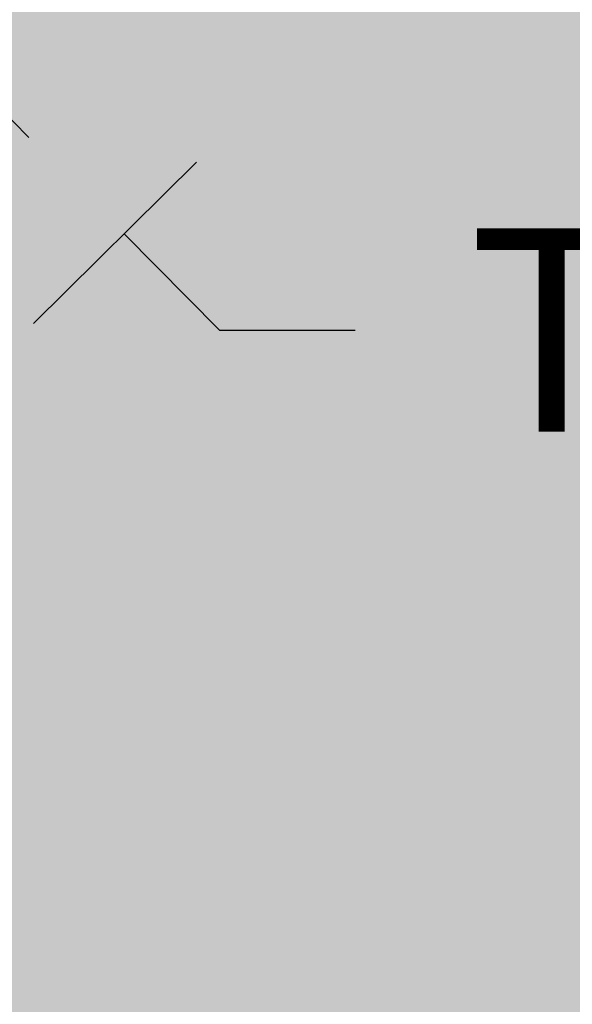
# Model space of a CAD drawing. Units: inches. Extents: x -466983 to 1020, y 324 to 318697.
# Tile 14 of 97: x 736 to 752, y 452 to 482. Entities that reach past the tile are written whole.
import ezdxf

# ---------------------------------------------------------------- set-up
doc = ezdxf.new("R2010")
doc.units = ezdxf.units.IN
doc.header["$MEASUREMENT"] = 0
doc.layers.add('A-ANNO-DIMS', color=2, linetype='Continuous', lineweight=18)
doc.layers.add('A-FLOR-PATT', color=252, linetype='Continuous', lineweight=13)
doc.styles.get("Standard").update_dxf_attribs({"font": 'arial.ttf'})
doc.dimstyles.get("Standard").update_dxf_attribs({"dimtxt": 6, "dimasz": 4, "dimexe": 3, "dimexo": 3, "dimgap": 0.09, "dimtad": 0, "dimtih": 1, "dimtoh": 1, "dimdec": 1, "dimzin": 0, "dimdsep": 46, "dimlunit": 3, "dimtxsty": 'Standard', "dimcen": 0.09, "dimadec": 0, "dimazin": 0, "dimtfac": 1, "dimtdec": 1, "dimtofl": 0, "dimtmove": 0, "dimatfit": 3, "dimfxl": 1, "dimtolj": 1, "dimtzin": 0, "dimarcsym": 0})

# ---------------------------------------------------------------- blocks, each defined once
blk = doc.blocks.new('*D113')
at = {"layer": 'A-ANNO-DIMS', "color": 0, "lineweight": -2, "transparency": 16777216}
for p, q in [((704.7099345407843, 504.6522237351473), (709.5248847709719, 509.4132675549068)), ((710.2041170385384, 504.4596180389745), (736.3194883324882, 478.0485582412536)), ((736.4502266725144, 472.5525555338968), (741.2651769027019, 477.3135993536564)), ((739.1319487513783, 475.2042540394889), (741.9444091702684, 472.359949837724)), ((741.9444091702684, 472.359949837724), (745.9444091702684, 472.359949837724))]:
    blk.add_line(p, q, dxfattribs=at)
at = {"layer": 'A-ANNO-DIMS', "color": 0, "transparency": 16777216}
for points in [[(710.6781677388324, 504.9283614421228), (709.7300663382443, 503.9908746358262), (707.3916566196483, 507.3039222407393)], [(736.7935390327824, 478.5173016444019), (735.8454376321941, 477.5798148381053), (739.1319487513783, 475.2042540394889)]]:
    blk.add_solid(points, dxfattribs=at)
at = {"layer": 'Defpoints', "color": 0, "transparency": 16777216}
for p in [(702.5767063894607, 502.5428784209798), (739.1319487513783, 475.2042540394889), (734.3169985211908, 470.4432102197293)]:
    blk.add_point(p, dxfattribs=at)
at = {"layer": 'A-ANNO-DIMS', "color": 0, "transparency": 16777216, "insert": (783.5016670147431, 472.359949837724), "char_height": 6, "attachment_point": 5}
blk.add_mtext('\\A1;TEA TABLE SET 45', dxfattribs=at)

msp = doc.modelspace()

# ---------------------------------------------------------------- hatches: boundary and pattern name
at = {"layer": 'A-FLOR-PATT', "transparency": 33554661}
h = msp.add_hatch(color=256, dxfattribs=at)
h.dxf.hatch_style = 1
h.set_gradient(color1=(19, 155, 72), color2=(0, 107, 0), name='CYLINDER')
h.paths.add_polyline_path([(813.8056775209042, 503.9377328184218), (730.8056775209043, 503.9377328184218), (730.8056775209043, 424.9377328184218), (612.8056775209042, 424.9377328184218), (612.8056775209042, 415.9377328184218), (442.8056775209042, 415.9377328184218), (442.8056775209042, 368.9377328184219), (813.8056775209042, 368.9377328184219)])
h.paths.add_polyline_path([(771.7959187717115, 407.069553802904), (783.7959187717115, 407.069553802904), (783.7959187717115, 371.069553802904), (771.7959187717115, 371.069553802904)], flags=16)
h.paths.add_polyline_path([(755.7959187717115, 407.069553802904), (755.7959187717115, 371.069553802904), (743.7959187717114, 371.069553802904), (743.7959187717114, 407.069553802904)], flags=16)
h.paths.add_polyline_path([(769.7959187717115, 404.069553802904), (769.7959187717115, 374.069553802904), (757.7959187717115, 374.069553802904), (757.7959187717115, 404.069553802904)], flags=16)
h.paths.add_polyline_path([(785.7959187717114, 404.069553802904), (797.7959187717114, 404.069553802904), (797.7959187717114, 374.069553802904), (785.7959187717114, 374.069553802904)], flags=16)
h.paths.add_polyline_path([(741.7959187717115, 404.069553802904), (741.7959187717115, 374.069553802904), (729.7959187717115, 374.069553802904), (729.7959187717115, 404.069553802904)], flags=16)
h.paths.add_polyline_path([(799.7959187717115, 407.069553802904), (811.7959187717115, 407.069553802904), (811.7959187717115, 371.069553802904), (799.7959187717115, 371.069553802904)], flags=16)
h.paths.add_polyline_path([(727.7959187717115, 407.069553802904), (727.7959187717115, 371.069553802904), (715.7959187717115, 371.069553802904), (715.7959187717115, 407.069553802904)], flags=16)
h.paths.add_polyline_path([(713.7959187717115, 404.069553802904), (713.7959187717115, 374.069553802904), (701.7959187717115, 374.069553802904), (701.7959187717115, 404.069553802904)], flags=16)
h.paths.add_polyline_path([(699.7959187717115, 407.069553802904), (699.7959187717115, 371.069553802904), (687.7959187717115, 371.069553802904), (687.7959187717115, 407.069553802904)], flags=16)
h.paths.add_polyline_path([(685.7959187717114, 404.069553802904), (685.7959187717114, 374.069553802904), (673.7959187717115, 374.069553802904), (673.7959187717115, 404.069553802904)], flags=16)
h.paths.add_polyline_path([(671.7959187717115, 407.069553802904), (671.7959187717115, 371.069553802904), (659.7959187717115, 371.069553802904), (659.7959187717115, 407.069553802904)], flags=16)
h.paths.add_polyline_path([(657.7959187717115, 404.069553802904), (657.7959187717115, 374.069553802904), (645.7959187717115, 374.069553802904), (645.7959187717115, 404.069553802904)], flags=16)
h.paths.add_polyline_path([(643.7959187717114, 407.069553802904), (643.7959187717114, 371.069553802904), (631.7959187717114, 371.069553802904), (631.7959187717114, 407.069553802904)], flags=16)
h.paths.add_polyline_path([(629.7959187717115, 404.069553802904), (629.7959187717115, 374.069553802904), (617.7959187717115, 374.069553802904), (617.7959187717115, 404.069553802904)], flags=16)
h.paths.add_polyline_path([(615.7959187717115, 407.069553802904), (615.7959187717115, 371.069553802904), (603.7959187717115, 371.069553802904), (603.7959187717115, 407.069553802904)], flags=16)
h.paths.add_polyline_path([(601.7959187717115, 404.069553802904), (601.7959187717115, 374.069553802904), (589.7959187717114, 374.069553802904), (589.7959187717114, 404.069553802904)], flags=16)
at = {"layer": 'A-FLOR-PATT'}
h = msp.add_hatch(dxfattribs=at)
h.set_pattern_fill('GRASS', color=256, scale=6)
h.set_pattern_definition([(90, (-1212.413693079869, -290.0350025265127), (-4.242640685999999, 4.242640685999999), [1.125, -7.360281377999999]), (45, (-1212.413693079869, -290.0350025265127), (-4.242640687119285, 4.242640687119285), [1.125, -4.875]), (135, (-1212.413693079869, -290.0350025265127), (-4.242640687119285, -4.242640687119284), [1.125, -4.875])])
h.paths.add_polyline_path([(813.8056775209042, 503.9377328184218), (730.8056775209043, 503.9377328184218), (730.8056775209043, 424.9377328184218), (612.8056775209042, 424.9377328184218), (612.8056775209042, 415.9377328184218), (442.8056775209042, 415.9377328184218), (442.8056775209042, 368.9377328184219), (813.8056775209042, 368.9377328184219)])
h.paths.add_polyline_path([(589.7959187717114, 404.069553802904), (601.7959187717115, 404.069553802904), (601.7959187717115, 374.069553802904), (589.7959187717114, 374.069553802904)], flags=16)
h.paths.add_polyline_path([(603.7959187717115, 407.069553802904), (615.7959187717115, 407.069553802904), (615.7959187717115, 371.069553802904), (603.7959187717115, 371.069553802904)], flags=16)
h.paths.add_polyline_path([(617.7959187717115, 404.069553802904), (629.7959187717115, 404.069553802904), (629.7959187717115, 374.069553802904), (617.7959187717115, 374.069553802904)], flags=16)
h.paths.add_polyline_path([(631.7959187717114, 407.069553802904), (643.7959187717114, 407.069553802904), (643.7959187717114, 371.069553802904), (631.7959187717114, 371.069553802904)], flags=16)
h.paths.add_polyline_path([(645.7959187717115, 404.069553802904), (657.7959187717115, 404.069553802904), (657.7959187717115, 374.069553802904), (645.7959187717115, 374.069553802904)], flags=16)
h.paths.add_polyline_path([(659.7959187717115, 407.069553802904), (671.7959187717115, 407.069553802904), (671.7959187717115, 371.069553802904), (659.7959187717115, 371.069553802904)], flags=16)
h.paths.add_polyline_path([(673.7959187717115, 404.069553802904), (685.7959187717114, 404.069553802904), (685.7959187717114, 374.069553802904), (673.7959187717115, 374.069553802904)], flags=16)
h.paths.add_polyline_path([(687.7959187717115, 407.069553802904), (699.7959187717115, 407.069553802904), (699.7959187717115, 371.069553802904), (687.7959187717115, 371.069553802904)], flags=16)
h.paths.add_polyline_path([(701.7959187717115, 404.069553802904), (713.7959187717115, 404.069553802904), (713.7959187717115, 374.069553802904), (701.7959187717115, 374.069553802904)], flags=16)
h.paths.add_polyline_path([(715.7959187717115, 407.069553802904), (727.7959187717115, 407.069553802904), (727.7959187717115, 371.069553802904), (715.7959187717115, 371.069553802904)], flags=16)
h.paths.add_polyline_path([(729.7959187717115, 404.069553802904), (741.7959187717115, 404.069553802904), (741.7959187717115, 374.069553802904), (729.7959187717115, 374.069553802904)], flags=16)
h.paths.add_polyline_path([(743.7959187717114, 407.069553802904), (755.7959187717115, 407.069553802904), (755.7959187717115, 371.069553802904), (743.7959187717114, 371.069553802904)], flags=16)
h.paths.add_polyline_path([(757.7959187717115, 404.069553802904), (769.7959187717115, 404.069553802904), (769.7959187717115, 374.069553802904), (757.7959187717115, 374.069553802904)], flags=16)
h.paths.add_polyline_path([(771.7959187717115, 407.069553802904), (783.7959187717115, 407.069553802904), (783.7959187717115, 371.069553802904), (771.7959187717115, 371.069553802904)], flags=16)
h.paths.add_polyline_path([(785.7959187717114, 404.069553802904), (797.7959187717114, 404.069553802904), (797.7959187717114, 374.069553802904), (785.7959187717114, 374.069553802904)], flags=16)
h.paths.add_polyline_path([(799.7959187717115, 407.069553802904), (811.7959187717115, 407.069553802904), (811.7959187717115, 371.069553802904), (799.7959187717115, 371.069553802904)], flags=16)

# ---------------------------------------------------------------- dimensions: what is measured, and where the dimension line sits
at = {"layer": 'A-ANNO-DIMS'}
dim = msp.add_linear_dim(base=(739.1319487513783, 475.2042540394889), p1=(702.5767063894607, 502.5428784209797), p2=(734.3169985211907, 470.4432102197293), angle=314.6774666770457, text='TEA TABLE SET <>', dimstyle='Standard', override={"dimdec": 0, "dimlfac": 1, "dimrnd": 0, "dimzin": 0, "dimdsep": 46, "dimlunit": 2}, dxfattribs=at)
dim.commit()
dim.dimension.update_dxf_attribs({"geometry": '*D113', "text_midpoint": (783.5016670147431, 472.359949837724)})

doc.saveas('drawing.dxf')
